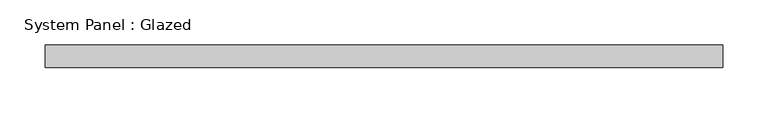
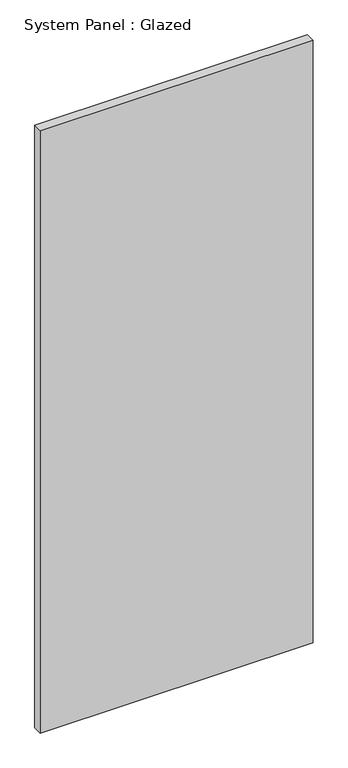
"""IFC4 building model written with IfcOpenShell, lengths in millimetres: plate geometry, System Panel : Glazed."""

from ifc_helpers import new_model, si_unit, origin, origin_with_axes, place, context, project, spatial, polyline, outline, extrude, source, transform, mapped, element, save


def system_panel_glazed_1e8a61fc(model_context):
    return source(origin(), model_context, "Body", "SweptSolid", [
        extrude(outline(polyline([(375.0, 24.5), (-375.0, 24.5), (-375.0, 49.5), (375.0, 49.5), (375.0, 24.5)])), origin_with_axes(), (0.0, 0.0, 1.0), 1750.0),
    ])


if __name__ == "__main__":
    model = new_model("IFC4")
    model_context = context("Model", 3, world=origin())
    ifc_project = project(units=[si_unit("LENGTHUNIT", "METRE", prefix="MILLI")], contexts=[model_context])
    site = spatial("IfcSite", under=ifc_project)
    building = spatial("IfcBuilding", under=site)
    placement = place(None, origin())
    system_panel_glazed_shape = system_panel_glazed_1e8a61fc(model_context)
    element("IfcPlate", 1, ObjectType="System Panel : Glazed", at=placement, inside=building, context=model_context, shape_type="MappedRepresentation", body=[
        mapped(system_panel_glazed_shape, transform((0.0, 0.0, 0.0), x_axis=(1.0, 0.0, 0.0), y_axis=(0.0, 1.0, 0.0), z_axis=(0.0, 0.0, 1.0))),
    ])
    save(model, "model.ifc")

# Revit data of these elements
# Type "System Panel : Glazed"
#   Construction Type Id = "GSP4R"
#   Analytic Construction = "1/8 in Pilkington single glazing"
#   Visual Light Transmittance = 0.9
#   Solar Heat Gain Coefficient = 0.86
#   Heat Transfer Coefficient (U) = 6.7069 W/(m²·K)
#   Define Thermal Properties by = 1
# Element 1 (IfcPlate, "System Panel : Glazed")
#   Materials on its faces: "Glass"
# Materials
#   "Glass": class "Glass", colour RGB 245 245 243, transparency 1, Description = "Soda Lime Glass", Cost = 0
